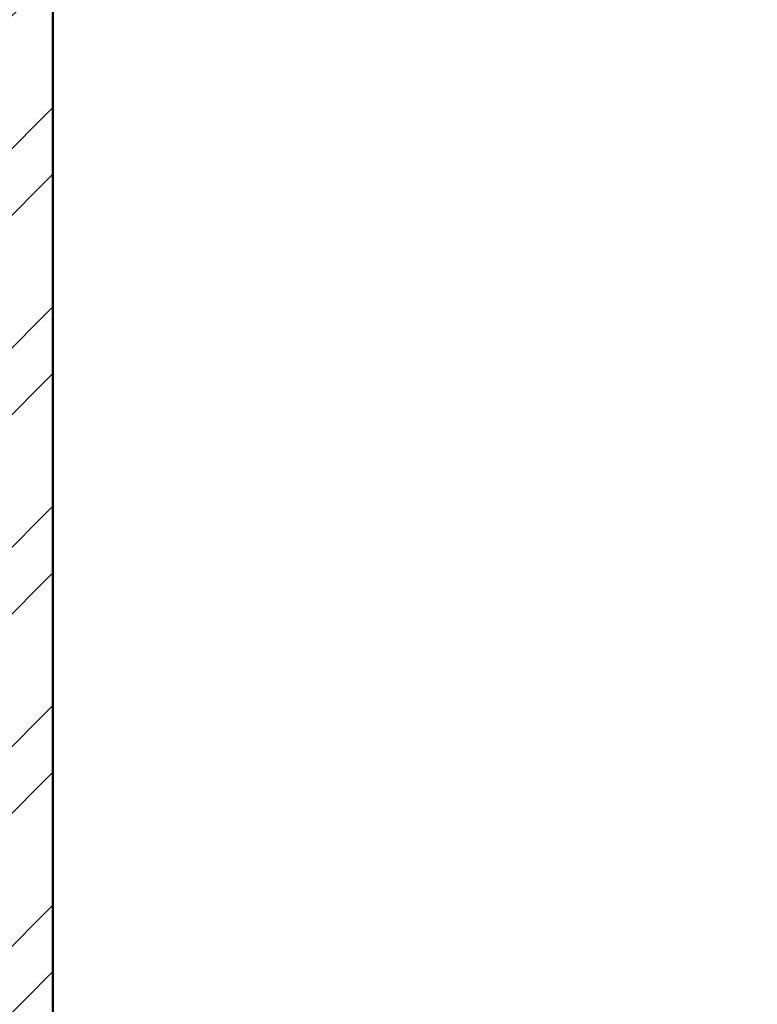
# Model space of a CAD drawing. Units: inches. Extents: x 963 to 2075, y 289 to 2657.
# Tile 6 of 98: x 1374 to 1424, y 1585 to 1652. Entities that reach past the tile are written whole.
import ezdxf

# ---------------------------------------------------------------- set-up
doc = ezdxf.new("R2010")
doc.units = ezdxf.units.IN
doc.layers.add('A-WALL', color=7, linetype='Continuous', lineweight=50)
doc.layers.add('A-WALL-PATT', color=8, linetype='Continuous', lineweight=13)

msp = doc.modelspace()

# ---------------------------------------------------------------- hatches: boundary and pattern name
at = {"layer": 'A-WALL-PATT'}
h = msp.add_hatch(dxfattribs=at)
h.set_pattern_fill('ANSI32', color=256)
h.paths.add_polyline_path([(1910.422, 1929.422), (1910.422, 1963.511), (1905.922, 1963.511), (1905.922, 1929.422), (1845.922, 1929.422), (1845.922, 1993.365), (1843.672, 1993.365), (1841.422, 1993.365), (1841.422, 1951.163), (1841.422, 1924.922), (1853.422, 1924.922), (1853.422, 1913.074), (1857.922, 1913.074), (1857.922, 1924.922), (1910.422, 1924.922)])
h.paths.add_polyline_path([(1857.922, 1853.074), (1853.422, 1853.074), (1853.422, 1826.318), (1841.422, 1826.318), (1674.482, 1826.318), (1674.482, 1821.818), (1853.422, 1821.818), (1857.922, 1821.818)])
h.paths.add_polyline_path([(1857.922, 1821.818), (1853.422, 1821.818), (1853.422, 1807.793), (1857.922, 1807.793)])
h.paths.add_polyline_path([(1857.922, 1747.793), (1853.422, 1747.793), (1853.422, 1713.818), (1809.343, 1713.818), (1809.343, 1709.318), (1905.922, 1709.318), (1905.922, 1688.318), (1910.422, 1688.318), (1910.422, 1713.818), (1857.922, 1713.818)])
h.paths.add_polyline_path([(1830.922, 1542.818), (1837.429, 1542.818), (1837.429, 1545.068), (1837.429, 1547.318), (1823.419, 1547.318), (1823.419, 1545.068), (1823.419, 1542.818), (1826.422, 1542.818), (1826.422, 1482.818), (1742.422, 1482.818), (1742.422, 1505.389), (1737.922, 1505.389), (1737.922, 1478.318), (1830.922, 1478.318)])
h.paths.add_polyline_path([(1938.922, 1619.318), (1934.422, 1619.318), (1910.422, 1619.318), (1910.422, 1628.318), (1908.172, 1628.318), (1905.922, 1628.318), (1905.922, 1614.818), (1934.422, 1614.818), (1934.422, 1547.318), (1905.922, 1547.318), (1899.589, 1547.318), (1899.589, 1542.818), (1910.422, 1542.818), (1938.922, 1542.818)])
h.paths.add_polyline_path([(1803.676, 1547.318), (1773.922, 1547.318), (1773.922, 1709.318), (1777.757, 1709.318), (1777.757, 1713.818), (1701.922, 1713.818), (1701.922, 1697.802), (1706.422, 1697.802), (1706.422, 1709.318), (1769.422, 1709.318), (1769.422, 1662.818), (1706.422, 1662.818), (1706.422, 1674.385), (1701.922, 1674.385), (1701.922, 1662.818), (1675.672, 1662.818), (1675.672, 1658.318), (1769.422, 1658.318), (1769.422, 1547.318), (1729.17, 1547.318), (1729.17, 1542.818), (1737.922, 1542.818), (1737.922, 1529.389), (1742.422, 1529.389), (1742.422, 1542.818), (1803.676, 1542.818)])
h.paths.add_polyline_path([(1595.422, 1542.818), (1599.245, 1542.818), (1599.245, 1547.318), (1584.36, 1547.318), (1584.36, 1542.818), (1590.922, 1542.818), (1590.922, 1436.318), (1595.422, 1436.318), (1595.422, 1440.818)])
h.paths.add_polyline_path([(1693.17, 1547.318), (1649.422, 1547.318), (1649.422, 1658.318), (1652.098, 1658.318), (1652.098, 1660.568), (1652.098, 1662.818), (1649.422, 1662.818), (1649.422, 1680.937), (1647.172, 1680.937), (1644.922, 1680.937), (1644.922, 1547.318), (1622.422, 1547.318), (1622.422, 1545.068), (1622.422, 1542.818), (1649.422, 1542.818), (1679.422, 1542.818), (1679.422, 1529.845), (1681.672, 1529.845), (1683.922, 1529.845), (1683.922, 1542.818), (1693.17, 1542.818), (1693.17, 1545.068)])
h.paths.add_polyline_path([(1683.922, 1505.845), (1679.422, 1505.845), (1679.422, 1483.805), (1595.422, 1483.805), (1595.422, 1479.305), (1683.922, 1479.305)])
h.paths.add_polyline_path([(1402.993, 1547.318), (1376.422, 1547.318), (1376.422, 1675.888), (1374.172, 1675.888), (1371.922, 1675.888), (1371.922, 1662.818), (1368.876, 1662.818), (1368.876, 1658.318), (1371.922, 1658.318), (1371.922, 1547.318), (1335.464, 1547.318), (1335.464, 1542.818), (1337.422, 1542.818), (1337.422, 1526.732), (1341.922, 1526.732), (1341.922, 1542.818), (1371.922, 1542.818), (1402.993, 1542.818)])

# ---------------------------------------------------------------- linework, layer by layer
at = {"layer": 'A-WALL'}
msp.add_line((1376.422, 1677.258), (1376.422, 1547.318), dxfattribs=at)

doc.saveas('drawing.dxf')
